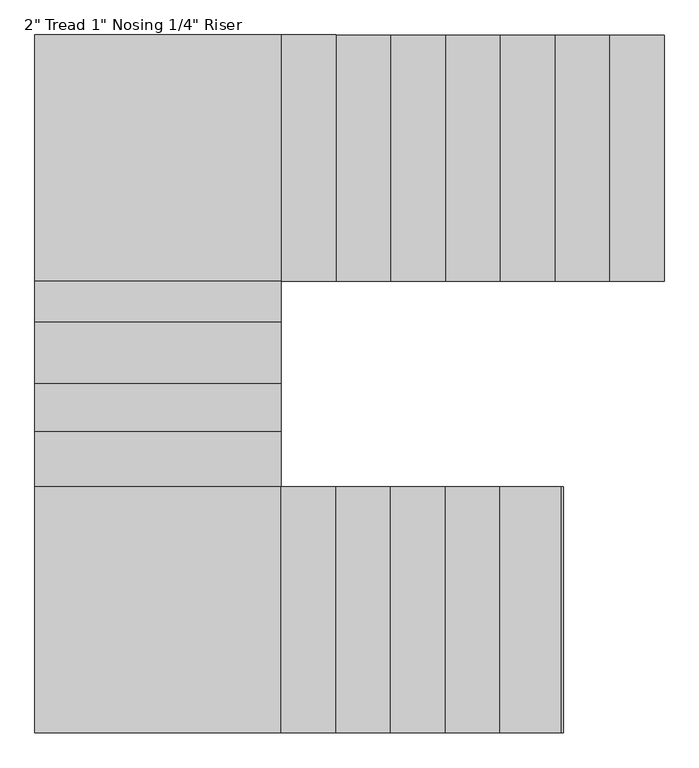
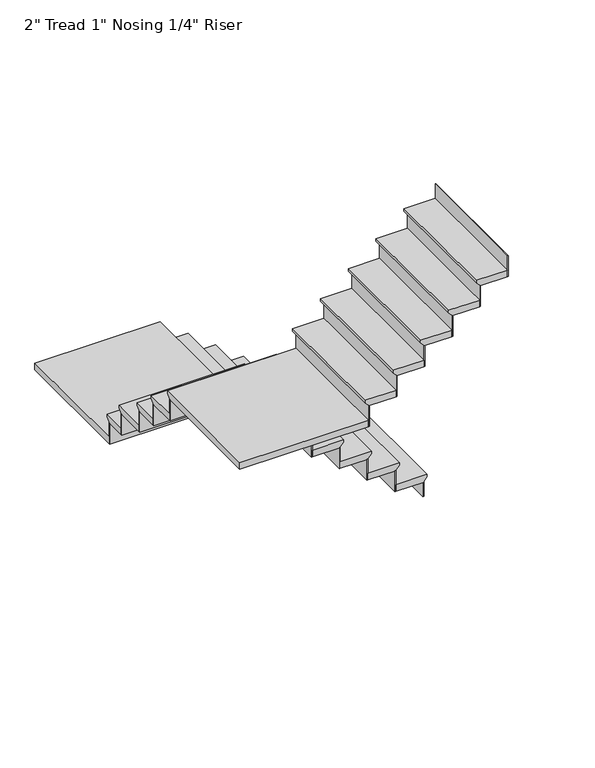
"""IFC4 building model written with IfcOpenShell, lengths in millimetres: stair flight geometry."""

from ifc_helpers import new_model, si_unit, origin, place, context, project, spatial, faceted_brep, source, transform, mapped, element, save


def stair_flight_50364206(model_context):
    return source(origin(), model_context, "Body", "Brep", [
        faceted_brep([(-3603.1340247, 922.0319954, 6542.1710526), (-3603.1340247, 922.0319954, 6561.2210526), (-3603.1340247, 7.6319954, 6561.2210526), (-3603.1340247, 7.6319954, 6542.1710526), (-3628.5340247, 922.0319954, 6516.7710526), (-3628.5340247, 7.6319954, 6516.7710526), (-3831.7340247, 922.0319954, 6561.2210526), (-3831.7340247, 7.6319954, 6561.2210526), (-3628.5340247, 7.6319954, 6510.4210526), (-3831.7340247, 7.6319954, 6510.4210526), (-3831.7340247, 922.0319954, 6510.4210526), (-3628.5340247, 922.0319954, 6510.4210526)], [[[0, 1, 2, 3]], [[4, 0, 3, 5]], [[2, 1, 6, 7]], [[8, 9, 10, 11]], [[2, 7, 9, 8, 5, 3]], [[8, 11, 4, 5]], [[6, 1, 0, 4, 11, 10]], [[7, 6, 10, 9]]]),
        faceted_brep([(-3628.5340247, 922.0319954, 6510.4210526), (-3628.5340247, 922.0319954, 6400.8), (-3634.8840247, 922.0319954, 6400.8), (-3634.8840247, 922.0319954, 6510.4210526), (-3628.5340247, 7.6319954, 6510.4210526), (-3634.8840247, 7.6319954, 6510.4210526), (-3634.8840247, 7.6319954, 6400.8), (-3628.5340247, 7.6319954, 6400.8)], [[[0, 1, 2, 3]], [[4, 5, 6, 7]], [[1, 0, 4, 7]], [[2, 1, 7, 6]], [[3, 2, 6, 5]], [[0, 3, 5, 4]]]),
        faceted_brep([(-3831.7340247, 922.0319954, 6670.8421053), (-3831.7340247, 922.0319954, 6510.4210526), (-3838.0840247, 922.0319954, 6510.4210526), (-3838.0840247, 922.0319954, 6670.8421053), (-3831.7340247, 7.6319954, 6670.8421053), (-3838.0840247, 7.6319954, 6670.8421053), (-3838.0840247, 7.6319954, 6510.4210526), (-3831.7340247, 7.6319954, 6510.4210526)], [[[0, 1, 2, 3]], [[4, 5, 6, 7]], [[1, 0, 4, 7]], [[2, 1, 7, 6]], [[3, 2, 6, 5]], [[0, 3, 5, 4]]]),
        faceted_brep([(-3806.3340247, 7.6319954, 6721.6421053), (-3806.3340247, 922.0319954, 6721.6421053), (-4034.9340247, 922.0319954, 6721.6421053), (-4034.9340247, 7.6319954, 6721.6421053), (-3831.7340247, 7.6319954, 6670.8421053), (-4034.9340247, 7.6319954, 6670.8421053), (-4034.9340247, 922.0319954, 6670.8421053), (-3831.7340247, 922.0319954, 6670.8421053), (-3831.7340247, 7.6319954, 6677.1921053), (-3806.3340247, 7.6319954, 6702.5921053), (-3831.7340247, 922.0319954, 6677.1921053), (-3806.3340247, 922.0319954, 6702.5921053)], [[[0, 1, 2, 3]], [[4, 5, 6, 7]], [[0, 3, 5, 4, 8, 9]], [[4, 7, 10, 8]], [[2, 1, 11, 10, 7, 6]], [[3, 2, 6, 5]], [[11, 1, 0, 9]], [[10, 11, 9, 8]]]),
        faceted_brep([(-4034.9340247, 922.0319954, 6831.2631579), (-4034.9340247, 922.0319954, 6670.8421053), (-4041.2840247, 922.0319954, 6670.8421053), (-4041.2840247, 922.0319954, 6831.2631579), (-4034.9340247, 7.6319954, 6831.2631579), (-4041.2840247, 7.6319954, 6831.2631579), (-4041.2840247, 7.6319954, 6670.8421053), (-4034.9340247, 7.6319954, 6670.8421053)], [[[0, 1, 2, 3]], [[4, 5, 6, 7]], [[1, 0, 4, 7]], [[2, 1, 7, 6]], [[3, 2, 6, 5]], [[0, 3, 5, 4]]]),
        faceted_brep([(-4009.5340247, 7.6319954, 6882.0631579), (-4009.5340247, 922.0319954, 6882.0631579), (-4238.1340247, 922.0319954, 6882.0631579), (-4238.1340247, 7.6319954, 6882.0631579), (-4034.9340247, 7.6319954, 6831.2631579), (-4238.1340247, 7.6319954, 6831.2631579), (-4238.1340247, 922.0319954, 6831.2631579), (-4034.9340247, 922.0319954, 6831.2631579), (-4034.9340247, 7.6319954, 6837.6131579), (-4009.5340247, 7.6319954, 6863.0131579), (-4034.9340247, 922.0319954, 6837.6131579), (-4009.5340247, 922.0319954, 6863.0131579)], [[[0, 1, 2, 3]], [[4, 5, 6, 7]], [[0, 3, 5, 4, 8, 9]], [[4, 7, 10, 8]], [[2, 1, 11, 10, 7, 6]], [[3, 2, 6, 5]], [[11, 1, 0, 9]], [[10, 11, 9, 8]]]),
        faceted_brep([(-4238.1340247, 922.0319954, 6991.6842105), (-4238.1340247, 922.0319954, 6831.2631579), (-4244.4840247, 922.0319954, 6831.2631579), (-4244.4840247, 922.0319954, 6991.6842105), (-4238.1340247, 7.6319954, 6991.6842105), (-4244.4840247, 7.6319954, 6991.6842105), (-4244.4840247, 7.6319954, 6831.2631579), (-4238.1340247, 7.6319954, 6831.2631579)], [[[0, 1, 2, 3]], [[4, 5, 6, 7]], [[1, 0, 4, 7]], [[2, 1, 7, 6]], [[3, 2, 6, 5]], [[0, 3, 5, 4]]]),
        faceted_brep([(-4212.7340247, 7.6319954, 7042.4842105), (-4212.7340247, 922.0319954, 7042.4842105), (-4441.3340247, 922.0319954, 7042.4842105), (-4441.3340247, 7.6319954, 7042.4842105), (-4238.1340247, 7.6319954, 6991.6842105), (-4441.3340247, 7.6319954, 6991.6842105), (-4441.3340247, 922.0319954, 6991.6842105), (-4238.1340247, 922.0319954, 6991.6842105), (-4238.1340247, 7.6319954, 6998.0342105), (-4212.7340247, 7.6319954, 7023.4342105), (-4238.1340247, 922.0319954, 6998.0342105), (-4212.7340247, 922.0319954, 7023.4342105)], [[[0, 1, 2, 3]], [[4, 5, 6, 7]], [[0, 3, 5, 4, 8, 9]], [[4, 7, 10, 8]], [[2, 1, 11, 10, 7, 6]], [[3, 2, 6, 5]], [[11, 1, 0, 9]], [[10, 11, 9, 8]]]),
        faceted_brep([(-4441.3340247, 922.0319954, 7152.1052632), (-4441.3340247, 922.0319954, 6991.6842105), (-4447.6840247, 922.0319954, 6991.6842105), (-4447.6840247, 922.0319954, 7152.1052632), (-4441.3340247, 7.6319954, 7152.1052632), (-4447.6840247, 7.6319954, 7152.1052632), (-4447.6840247, 7.6319954, 6991.6842105), (-4441.3340247, 7.6319954, 6991.6842105)], [[[0, 1, 2, 3]], [[4, 5, 6, 7]], [[1, 0, 4, 7]], [[2, 1, 7, 6]], [[3, 2, 6, 5]], [[0, 3, 5, 4]]]),
        faceted_brep([(-4415.9340247, 7.6319954, 7202.9052632), (-4415.9340247, 922.0319954, 7202.9052632), (-4644.5340247, 922.0319954, 7202.9052632), (-4644.5340247, 7.6319954, 7202.9052632), (-4441.3340247, 7.6319954, 7152.1052632), (-4644.5340247, 7.6319954, 7152.1052632), (-4644.5340247, 922.0319954, 7152.1052632), (-4441.3340247, 922.0319954, 7152.1052632), (-4441.3340247, 7.6319954, 7158.4552632), (-4415.9340247, 7.6319954, 7183.8552632), (-4441.3340247, 922.0319954, 7158.4552632), (-4415.9340247, 922.0319954, 7183.8552632)], [[[0, 1, 2, 3]], [[4, 5, 6, 7]], [[0, 3, 5, 4, 8, 9]], [[4, 7, 10, 8]], [[2, 1, 11, 10, 7, 6]], [[3, 2, 6, 5]], [[11, 1, 0, 9]], [[10, 11, 9, 8]]]),
        faceted_brep([(-4644.5340247, 922.0319954, 7312.5263158), (-4644.5340247, 922.0319954, 7152.1052632), (-4650.8840247, 922.0319954, 7152.1052632), (-4650.8840247, 922.0319954, 7312.5263158), (-4644.5340247, 7.6319954, 7312.5263158), (-4650.8840247, 7.6319954, 7312.5263158), (-4650.8840247, 7.6319954, 7152.1052632), (-4644.5340247, 7.6319954, 7152.1052632)], [[[0, 1, 2, 3]], [[4, 5, 6, 7]], [[1, 0, 4, 7]], [[2, 1, 7, 6]], [[3, 2, 6, 5]], [[0, 3, 5, 4]]]),
        faceted_brep([(-4619.1340247, 7.6319954, 7363.3263158), (-4619.1340247, 922.0319954, 7363.3263158), (-4847.7340247, 922.0319954, 7363.3263158), (-4847.7340247, 7.6319954, 7363.3263158), (-4644.5340247, 7.6319954, 7312.5263158), (-4847.7340247, 7.6319954, 7312.5263158), (-4847.7340247, 922.0319954, 7312.5263158), (-4644.5340247, 922.0319954, 7312.5263158), (-4644.5340247, 7.6319954, 7318.8763158), (-4619.1340247, 7.6319954, 7344.2763158), (-4644.5340247, 922.0319954, 7318.8763158), (-4619.1340247, 922.0319954, 7344.2763158)], [[[0, 1, 2, 3]], [[4, 5, 6, 7]], [[0, 3, 5, 4, 8, 9]], [[4, 7, 10, 8]], [[2, 1, 11, 10, 7, 6]], [[3, 2, 6, 5]], [[11, 1, 0, 9]], [[10, 11, 9, 8]]]),
        faceted_brep([(-4847.7340247, 922.0319954, 7472.9473684), (-4847.7340247, 922.0319954, 7312.5263158), (-4854.0840247, 922.0319954, 7312.5263158), (-4854.0840247, 922.0319954, 7472.9473684), (-4847.7340247, 7.6319954, 7472.9473684), (-4854.0840247, 7.6319954, 7472.9473684), (-4854.0840247, 7.6319954, 7312.5263158), (-4847.7340247, 7.6319954, 7312.5263158)], [[[0, 1, 2, 3]], [[4, 5, 6, 7]], [[1, 0, 4, 7]], [[2, 1, 7, 6]], [[3, 2, 6, 5]], [[0, 3, 5, 4]]]),
        faceted_brep([(-4822.3340247, 7.6319954, 7523.7473684), (-4822.3340247, 922.0319954, 7523.7473684), (-5050.9340247, 922.0319954, 7523.7473684), (-5050.9340247, 7.6319954, 7523.7473684), (-4847.7340247, 7.6319954, 7472.9473684), (-5050.9340247, 7.6319954, 7472.9473684), (-5050.9340247, 922.0319954, 7472.9473684), (-4847.7340247, 922.0319954, 7472.9473684), (-4847.7340247, 7.6319954, 7479.2973684), (-4822.3340247, 7.6319954, 7504.6973684), (-4847.7340247, 922.0319954, 7479.2973684), (-4822.3340247, 922.0319954, 7504.6973684)], [[[0, 1, 2, 3]], [[4, 5, 6, 7]], [[0, 3, 5, 4, 8, 9]], [[4, 7, 10, 8]], [[2, 1, 11, 10, 7, 6]], [[3, 2, 6, 5]], [[11, 1, 0, 9]], [[10, 11, 9, 8]]]),
        faceted_brep([(-5050.9340247, 922.0319954, 7633.3684211), (-5050.9340247, 922.0319954, 7472.9473684), (-5057.2840247, 922.0319954, 7472.9473684), (-5057.2840247, 922.0319954, 7633.3684211), (-5050.9340247, 7.6319954, 7633.3684211), (-5057.2840247, 7.6319954, 7633.3684211), (-5057.2840247, 7.6319954, 7472.9473684), (-5050.9340247, 7.6319954, 7472.9473684)], [[[0, 1, 2, 3]], [[4, 5, 6, 7]], [[1, 0, 4, 7]], [[2, 1, 7, 6]], [[3, 2, 6, 5]], [[0, 3, 5, 4]]]),
        faceted_brep([(-5939.9340247, 922.0319954, 7684.1684211), (-5939.9340247, -17.7680046, 7684.1684211), (-5025.5340247, -17.7680046, 7684.1684211), (-5025.5340247, 922.0319954, 7684.1684211), (-5025.5340247, 7.6319954, 7633.3684211), (-5025.5340247, -17.7680046, 7633.3684211), (-5939.9340247, -17.7680046, 7633.3684211), (-5939.9340247, 922.0319954, 7633.3684211), (-5050.9340247, 922.0319954, 7633.3684211), (-5050.9340247, 7.6319954, 7633.3684211), (-5025.5340247, 7.6319954, 7665.1184211), (-5025.5340247, 922.0319954, 7665.1184211), (-5050.9340247, 7.6319954, 7639.7184211), (-5050.9340247, 922.0319954, 7639.7184211)], [[[0, 1, 2, 3]], [[4, 5, 6, 7, 8, 9]], [[3, 2, 5, 4, 10, 11]], [[4, 9, 12, 10]], [[9, 8, 13, 12]], [[0, 3, 11, 13, 8, 7]], [[1, 0, 7, 6]], [[2, 1, 6, 5]], [[13, 11, 10, 12]]]),
        faceted_brep([(-5939.9340247, -17.7680046, 7793.7894737), (-5939.9340247, -17.7680046, 7633.3684211), (-5939.9340247, -24.1180046, 7633.3684211), (-5939.9340247, -24.1180046, 7793.7894737), (-5025.5340247, -17.7680046, 7793.7894737), (-5025.5340247, -24.1180046, 7793.7894737), (-5025.5340247, -24.1180046, 7633.3684211), (-5025.5340247, -17.7680046, 7633.3684211)], [[[0, 1, 2, 3]], [[4, 5, 6, 7]], [[1, 0, 4, 7]], [[2, 1, 7, 6]], [[3, 2, 6, 5]], [[0, 3, 5, 4]]]),
        faceted_brep([(-5025.5340247, 7.6319954, 7844.5894737), (-5939.9340247, 7.6319954, 7844.5894737), (-5939.9340247, -170.1680046, 7844.5894737), (-5025.5340247, -170.1680046, 7844.5894737), (-5025.5340247, -17.7680046, 7793.7894737), (-5025.5340247, -170.1680046, 7793.7894737), (-5939.9340247, -170.1680046, 7793.7894737), (-5939.9340247, -17.7680046, 7793.7894737), (-5025.5340247, -17.7680046, 7800.1394737), (-5025.5340247, 7.6319954, 7825.5394737), (-5939.9340247, -17.7680046, 7800.1394737), (-5939.9340247, 7.6319954, 7825.5394737)], [[[0, 1, 2, 3]], [[4, 5, 6, 7]], [[0, 3, 5, 4, 8, 9]], [[4, 7, 10, 8]], [[2, 1, 11, 10, 7, 6]], [[3, 2, 6, 5]], [[11, 1, 0, 9]], [[10, 11, 9, 8]]]),
        faceted_brep([(-5939.9340247, -170.1680046, 7954.2105263), (-5939.9340247, -170.1680046, 7793.7894737), (-5939.9340247, -176.5180046, 7793.7894737), (-5939.9340247, -176.5180046, 7954.2105263), (-5025.5340247, -170.1680046, 7954.2105263), (-5025.5340247, -176.5180046, 7954.2105263), (-5025.5340247, -176.5180046, 7793.7894737), (-5025.5340247, -170.1680046, 7793.7894737)], [[[0, 1, 2, 3]], [[4, 5, 6, 7]], [[1, 0, 4, 7]], [[2, 1, 7, 6]], [[3, 2, 6, 5]], [[0, 3, 5, 4]]]),
        faceted_brep([(-5025.5340247, -144.7680046, 8005.0105263), (-5939.9340247, -144.7680046, 8005.0105263), (-5939.9340247, -398.7680046, 8005.0105263), (-5025.5340247, -398.7680046, 8005.0105263), (-5025.5340247, -170.1680046, 7954.2105263), (-5025.5340247, -398.7680046, 7954.2105263), (-5939.9340247, -398.7680046, 7954.2105263), (-5939.9340247, -170.1680046, 7954.2105263), (-5025.5340247, -170.1680046, 7960.5605263), (-5025.5340247, -144.7680046, 7985.9605263), (-5939.9340247, -170.1680046, 7960.5605263), (-5939.9340247, -144.7680046, 7985.9605263)], [[[0, 1, 2, 3]], [[4, 5, 6, 7]], [[0, 3, 5, 4, 8, 9]], [[4, 7, 10, 8]], [[2, 1, 11, 10, 7, 6]], [[3, 2, 6, 5]], [[11, 1, 0, 9]], [[10, 11, 9, 8]]]),
        faceted_brep([(-5939.9340247, -398.7680046, 8114.6315789), (-5939.9340247, -398.7680046, 7954.2105263), (-5939.9340247, -405.1180046, 7954.2105263), (-5939.9340247, -405.1180046, 8114.6315789), (-5025.5340247, -398.7680046, 8114.6315789), (-5025.5340247, -405.1180046, 8114.6315789), (-5025.5340247, -405.1180046, 7954.2105263), (-5025.5340247, -398.7680046, 7954.2105263)], [[[0, 1, 2, 3]], [[4, 5, 6, 7]], [[1, 0, 4, 7]], [[2, 1, 7, 6]], [[3, 2, 6, 5]], [[0, 3, 5, 4]]]),
        faceted_brep([(-5025.5340247, -373.3680046, 8165.4315789), (-5939.9340247, -373.3680046, 8165.4315789), (-5939.9340247, -576.5680046, 8165.4315789), (-5025.5340247, -576.5680046, 8165.4315789), (-5025.5340247, -398.7680046, 8114.6315789), (-5025.5340247, -576.5680046, 8114.6315789), (-5939.9340247, -576.5680046, 8114.6315789), (-5939.9340247, -398.7680046, 8114.6315789), (-5025.5340247, -398.7680046, 8120.9815789), (-5025.5340247, -373.3680046, 8146.3815789), (-5939.9340247, -398.7680046, 8120.9815789), (-5939.9340247, -373.3680046, 8146.3815789)], [[[0, 1, 2, 3]], [[4, 5, 6, 7]], [[0, 3, 5, 4, 8, 9]], [[4, 7, 10, 8]], [[2, 1, 11, 10, 7, 6]], [[3, 2, 6, 5]], [[11, 1, 0, 9]], [[10, 11, 9, 8]]]),
        faceted_brep([(-5939.9340247, -576.5680046, 8275.0526316), (-5939.9340247, -576.5680046, 8114.6315789), (-5939.9340247, -582.9180046, 8114.6315789), (-5939.9340247, -582.9180046, 8275.0526316), (-5025.5340247, -576.5680046, 8275.0526316), (-5025.5340247, -582.9180046, 8275.0526316), (-5025.5340247, -582.9180046, 8114.6315789), (-5025.5340247, -576.5680046, 8114.6315789)], [[[0, 1, 2, 3]], [[4, 5, 6, 7]], [[1, 0, 4, 7]], [[2, 1, 7, 6]], [[3, 2, 6, 5]], [[0, 3, 5, 4]]]),
        faceted_brep([(-5025.5340247, -551.1680046, 8325.8526316), (-5939.9340247, -551.1680046, 8325.8526316), (-5939.9340247, -779.7680046, 8325.8526316), (-5025.5340247, -779.7680046, 8325.8526316), (-5025.5340247, -576.5680046, 8275.0526316), (-5025.5340247, -779.7680046, 8275.0526316), (-5939.9340247, -779.7680046, 8275.0526316), (-5939.9340247, -576.5680046, 8275.0526316), (-5025.5340247, -576.5680046, 8281.4026316), (-5025.5340247, -551.1680046, 8306.8026316), (-5939.9340247, -576.5680046, 8281.4026316), (-5939.9340247, -551.1680046, 8306.8026316)], [[[0, 1, 2, 3]], [[4, 5, 6, 7]], [[0, 3, 5, 4, 8, 9]], [[4, 7, 10, 8]], [[2, 1, 11, 10, 7, 6]], [[3, 2, 6, 5]], [[11, 1, 0, 9]], [[10, 11, 9, 8]]]),
        faceted_brep([(-5939.9340247, -779.7680046, 8435.4736842), (-5939.9340247, -779.7680046, 8275.0526316), (-5939.9340247, -786.1180046, 8275.0526316), (-5939.9340247, -786.1180046, 8435.4736842), (-5025.5340247, -779.7680046, 8435.4736842), (-5025.5340247, -786.1180046, 8435.4736842), (-5025.5340247, -786.1180046, 8275.0526316), (-5025.5340247, -779.7680046, 8275.0526316)], [[[0, 1, 2, 3]], [[4, 5, 6, 7]], [[1, 0, 4, 7]], [[2, 1, 7, 6]], [[3, 2, 6, 5]], [[0, 3, 5, 4]]]),
        faceted_brep([(-5939.9340247, -1668.7680046, 8486.2736842), (-5000.1340247, -1668.7680046, 8486.2736842), (-5000.1340247, -754.3680046, 8486.2736842), (-5939.9340247, -754.3680046, 8486.2736842), (-5025.5340247, -754.3680046, 8435.4736842), (-5000.1340247, -754.3680046, 8435.4736842), (-5000.1340247, -1668.7680046, 8435.4736842), (-5939.9340247, -1668.7680046, 8435.4736842), (-5939.9340247, -779.7680046, 8435.4736842), (-5025.5340247, -779.7680046, 8435.4736842), (-5025.5340247, -754.3680046, 8467.2236842), (-5939.9340247, -754.3680046, 8467.2236842), (-5025.5340247, -779.7680046, 8441.8236842), (-5939.9340247, -779.7680046, 8441.8236842)], [[[0, 1, 2, 3]], [[4, 5, 6, 7, 8, 9]], [[3, 2, 5, 4, 10, 11]], [[4, 9, 12, 10]], [[9, 8, 13, 12]], [[0, 3, 11, 13, 8, 7]], [[1, 0, 7, 6]], [[2, 1, 6, 5]], [[13, 11, 10, 12]]]),
        faceted_brep([(-5000.1340247, -1668.7680046, 8595.8947368), (-5000.1340247, -1668.7680046, 8435.4736842), (-4993.7840247, -1668.7680046, 8435.4736842), (-4993.7840247, -1668.7680046, 8595.8947368), (-5000.1340247, -754.3680046, 8595.8947368), (-4993.7840247, -754.3680046, 8595.8947368), (-4993.7840247, -754.3680046, 8435.4736842), (-5000.1340247, -754.3680046, 8435.4736842)], [[[0, 1, 2, 3]], [[4, 5, 6, 7]], [[1, 0, 4, 7]], [[2, 1, 7, 6]], [[3, 2, 6, 5]], [[0, 3, 5, 4]]]),
        faceted_brep([(-5025.5340247, -754.3680046, 8646.6947368), (-5025.5340247, -1668.7680046, 8646.6947368), (-4796.9340247, -1668.7680046, 8646.6947368), (-4796.9340247, -754.3680046, 8646.6947368), (-5000.1340247, -754.3680046, 8595.8947368), (-4796.9340247, -754.3680046, 8595.8947368), (-4796.9340247, -1668.7680046, 8595.8947368), (-5000.1340247, -1668.7680046, 8595.8947368), (-5000.1340247, -754.3680046, 8602.2447368), (-5025.5340247, -754.3680046, 8627.6447368), (-5000.1340247, -1668.7680046, 8602.2447368), (-5025.5340247, -1668.7680046, 8627.6447368)], [[[0, 1, 2, 3]], [[4, 5, 6, 7]], [[0, 3, 5, 4, 8, 9]], [[4, 7, 10, 8]], [[2, 1, 11, 10, 7, 6]], [[3, 2, 6, 5]], [[11, 1, 0, 9]], [[10, 11, 9, 8]]]),
        faceted_brep([(-4796.9340247, -1668.7680046, 8756.3157895), (-4796.9340247, -1668.7680046, 8595.8947368), (-4790.5840247, -1668.7680046, 8595.8947368), (-4790.5840247, -1668.7680046, 8756.3157895), (-4796.9340247, -754.3680046, 8756.3157895), (-4790.5840247, -754.3680046, 8756.3157895), (-4790.5840247, -754.3680046, 8595.8947368), (-4796.9340247, -754.3680046, 8595.8947368)], [[[0, 1, 2, 3]], [[4, 5, 6, 7]], [[1, 0, 4, 7]], [[2, 1, 7, 6]], [[3, 2, 6, 5]], [[0, 3, 5, 4]]]),
        faceted_brep([(-4822.3340247, -754.3680046, 8807.1157895), (-4822.3340247, -1668.7680046, 8807.1157895), (-4593.7340247, -1668.7680046, 8807.1157895), (-4593.7340247, -754.3680046, 8807.1157895), (-4796.9340247, -754.3680046, 8756.3157895), (-4593.7340247, -754.3680046, 8756.3157895), (-4593.7340247, -1668.7680046, 8756.3157895), (-4796.9340247, -1668.7680046, 8756.3157895), (-4796.9340247, -754.3680046, 8762.6657895), (-4822.3340247, -754.3680046, 8788.0657895), (-4796.9340247, -1668.7680046, 8762.6657895), (-4822.3340247, -1668.7680046, 8788.0657895)], [[[0, 1, 2, 3]], [[4, 5, 6, 7]], [[0, 3, 5, 4, 8, 9]], [[4, 7, 10, 8]], [[2, 1, 11, 10, 7, 6]], [[3, 2, 6, 5]], [[11, 1, 0, 9]], [[10, 11, 9, 8]]]),
        faceted_brep([(-4593.7340247, -1668.7680046, 8916.7368421), (-4593.7340247, -1668.7680046, 8756.3157895), (-4587.3840247, -1668.7680046, 8756.3157895), (-4587.3840247, -1668.7680046, 8916.7368421), (-4593.7340247, -754.3680046, 8916.7368421), (-4587.3840247, -754.3680046, 8916.7368421), (-4587.3840247, -754.3680046, 8756.3157895), (-4593.7340247, -754.3680046, 8756.3157895)], [[[0, 1, 2, 3]], [[4, 5, 6, 7]], [[1, 0, 4, 7]], [[2, 1, 7, 6]], [[3, 2, 6, 5]], [[0, 3, 5, 4]]]),
        faceted_brep([(-4619.1340247, -754.3680046, 8967.5368421), (-4619.1340247, -1668.7680046, 8967.5368421), (-4390.5340247, -1668.7680046, 8967.5368421), (-4390.5340247, -754.3680046, 8967.5368421), (-4593.7340247, -754.3680046, 8916.7368421), (-4390.5340247, -754.3680046, 8916.7368421), (-4390.5340247, -1668.7680046, 8916.7368421), (-4593.7340247, -1668.7680046, 8916.7368421), (-4593.7340247, -754.3680046, 8923.0868421), (-4619.1340247, -754.3680046, 8948.4868421), (-4593.7340247, -1668.7680046, 8923.0868421), (-4619.1340247, -1668.7680046, 8948.4868421)], [[[0, 1, 2, 3]], [[4, 5, 6, 7]], [[0, 3, 5, 4, 8, 9]], [[4, 7, 10, 8]], [[2, 1, 11, 10, 7, 6]], [[3, 2, 6, 5]], [[11, 1, 0, 9]], [[10, 11, 9, 8]]]),
        faceted_brep([(-4390.5340247, -1668.7680046, 9077.1578947), (-4390.5340247, -1668.7680046, 8916.7368421), (-4384.1840247, -1668.7680046, 8916.7368421), (-4384.1840247, -1668.7680046, 9077.1578947), (-4390.5340247, -754.3680046, 9077.1578947), (-4384.1840247, -754.3680046, 9077.1578947), (-4384.1840247, -754.3680046, 8916.7368421), (-4390.5340247, -754.3680046, 8916.7368421)], [[[0, 1, 2, 3]], [[4, 5, 6, 7]], [[1, 0, 4, 7]], [[2, 1, 7, 6]], [[3, 2, 6, 5]], [[0, 3, 5, 4]]]),
        faceted_brep([(-4415.9340247, -754.3680046, 9127.9578947), (-4415.9340247, -1668.7680046, 9127.9578947), (-4187.3340247, -1668.7680046, 9127.9578947), (-4187.3340247, -754.3680046, 9127.9578947), (-4390.5340247, -754.3680046, 9077.1578947), (-4187.3340247, -754.3680046, 9077.1578947), (-4187.3340247, -1668.7680046, 9077.1578947), (-4390.5340247, -1668.7680046, 9077.1578947), (-4390.5340247, -754.3680046, 9083.5078947), (-4415.9340247, -754.3680046, 9108.9078947), (-4390.5340247, -1668.7680046, 9083.5078947), (-4415.9340247, -1668.7680046, 9108.9078947)], [[[0, 1, 2, 3]], [[4, 5, 6, 7]], [[0, 3, 5, 4, 8, 9]], [[4, 7, 10, 8]], [[2, 1, 11, 10, 7, 6]], [[3, 2, 6, 5]], [[11, 1, 0, 9]], [[10, 11, 9, 8]]]),
        faceted_brep([(-4187.3340247, -1668.7680046, 9237.5789474), (-4187.3340247, -1668.7680046, 9077.1578947), (-4180.9840247, -1668.7680046, 9077.1578947), (-4180.9840247, -1668.7680046, 9237.5789474), (-4187.3340247, -754.3680046, 9237.5789474), (-4180.9840247, -754.3680046, 9237.5789474), (-4180.9840247, -754.3680046, 9077.1578947), (-4187.3340247, -754.3680046, 9077.1578947)], [[[0, 1, 2, 3]], [[4, 5, 6, 7]], [[1, 0, 4, 7]], [[2, 1, 7, 6]], [[3, 2, 6, 5]], [[0, 3, 5, 4]]]),
        faceted_brep([(-3984.1340247, -1668.7680046, 9398.0), (-3984.1340247, -1668.7680046, 9237.5789474), (-3977.7840247, -1668.7680046, 9237.5789474), (-3977.7840247, -1668.7680046, 9398.0), (-3984.1340247, -754.3680046, 9398.0), (-3977.7840247, -754.3680046, 9398.0), (-3977.7840247, -754.3680046, 9237.5789474), (-3984.1340247, -754.3680046, 9237.5789474)], [[[0, 1, 2, 3]], [[4, 5, 6, 7]], [[1, 0, 4, 7]], [[2, 1, 7, 6]], [[3, 2, 6, 5]], [[0, 3, 5, 4]]]),
        faceted_brep([(-4212.7340247, -754.3680046, 9288.3789474), (-4212.7340247, -1668.7680046, 9288.3789474), (-3984.1340247, -1668.7680046, 9288.3789474), (-3984.1340247, -754.3680046, 9288.3789474), (-4187.3340247, -754.3680046, 9237.5789474), (-3984.1340247, -754.3680046, 9237.5789474), (-3984.1340247, -1668.7680046, 9237.5789474), (-4187.3340247, -1668.7680046, 9237.5789474), (-4187.3340247, -754.3680046, 9243.9289474), (-4212.7340247, -754.3680046, 9269.3289474), (-4187.3340247, -1668.7680046, 9243.9289474), (-4212.7340247, -1668.7680046, 9269.3289474)], [[[0, 1, 2, 3]], [[4, 5, 6, 7]], [[0, 3, 5, 4, 8, 9]], [[4, 7, 10, 8]], [[2, 1, 11, 10, 7, 6]], [[3, 2, 6, 5]], [[11, 1, 0, 9]], [[10, 11, 9, 8]]]),
    ])


if __name__ == "__main__":
    model = new_model("IFC4")
    model_context = context("Model", 3, world=origin())
    ifc_project = project(units=[si_unit("LENGTHUNIT", "METRE", prefix="MILLI")], contexts=[model_context])
    site = spatial("IfcSite", under=ifc_project)
    building = spatial("IfcBuilding", under=site)
    placement = place(None, origin())
    stair_flight_shape = stair_flight_50364206(model_context)
    element("IfcStairFlight", 1, ObjectType="2\" Tread 1\" Nosing 1/4\" Riser", at=placement, inside=building, context=model_context, shape_type="MappedRepresentation", body=[
        mapped(stair_flight_shape, transform((0.0, 0.0, 0.0), x_axis=(1.0, 0.0, 0.0), y_axis=(0.0, 1.0, 0.0), z_axis=(0.0, 0.0, 1.0))),
    ])
    save(model, "model.ifc")
